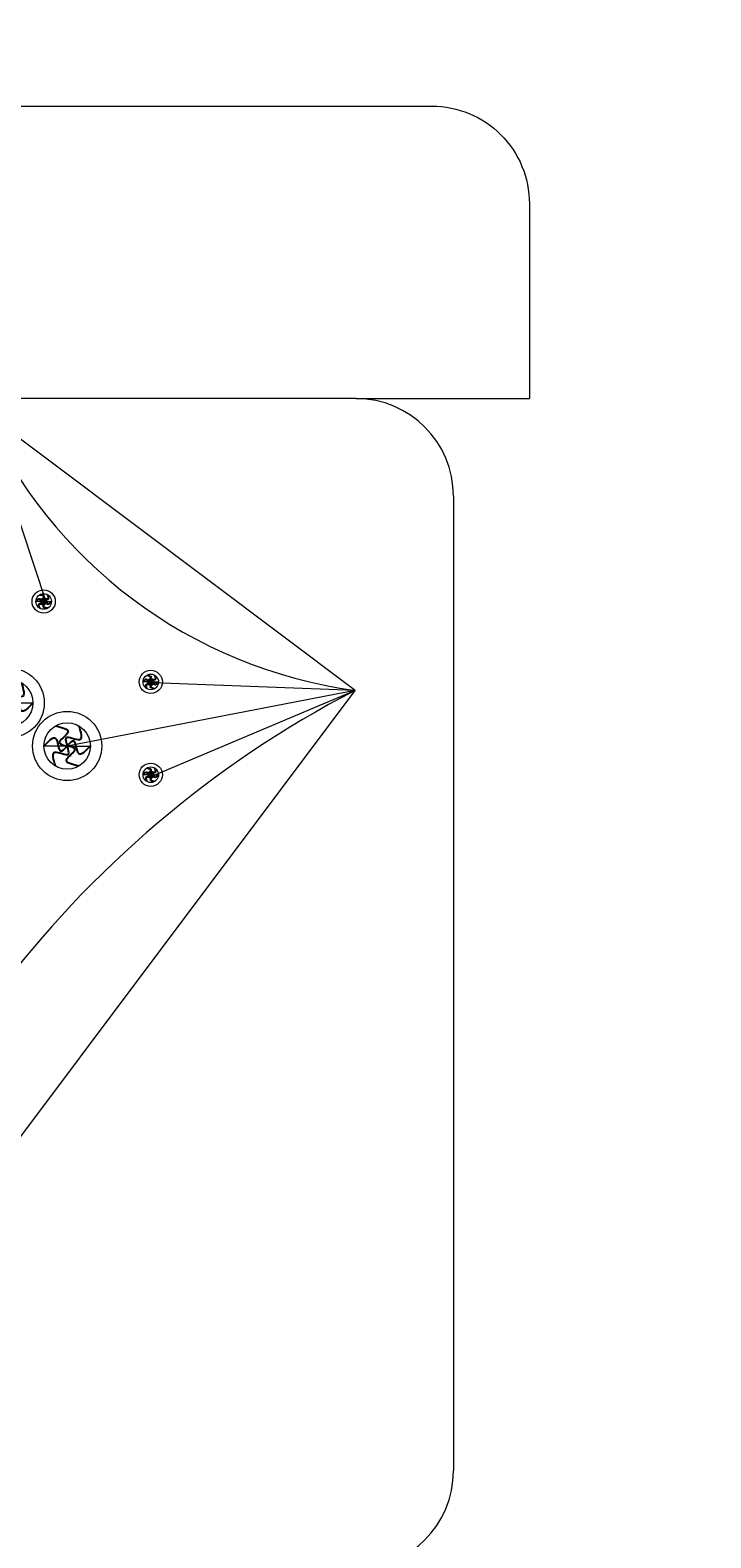
# Model space of a CAD drawing. Units: inches. Extents: x -61 to 1599, y -1316 to 257.
# Tile 105 of 204: x 142 to 156, y -99 to -68. Entities that reach past the tile are written whole.
import ezdxf

# ---------------------------------------------------------------- set-up
doc = ezdxf.new("R2010")
doc.units = ezdxf.units.IN
doc.header["$MEASUREMENT"] = 0
doc.layers.add('A-ANNO-DIMS', color=2, linetype='Continuous', lineweight=18)
doc.layers.add('FURNITURE', color=83, linetype='Continuous', lineweight=18)
doc.layers.add('FUR', color=83, linetype='Continuous')
doc.styles.get("Standard").update_dxf_attribs({"font": 'arial.ttf'})
doc.dimstyles.get("Standard").update_dxf_attribs({"dimtxt": 0.18, "dimasz": 0.18, "dimexe": 0.18, "dimexo": 0.0625, "dimgap": 0.09, "dimtad": 0, "dimtih": 1, "dimtoh": 1, "dimdec": 0, "dimzin": 0, "dimdsep": 46, "dimlunit": 3, "dimtxsty": 'Standard', "dimcen": 0.09, "dimadec": 0, "dimazin": 0, "dimtfac": 1, "dimtdec": 0, "dimtofl": 0, "dimtmove": 0, "dimatfit": 3, "dimfxl": 1, "dimtolj": 1, "dimtzin": 0, "dimarcsym": 0})

# ---------------------------------------------------------------- blocks, each defined once
blk = doc.blocks.new('*U209')
at = {"layer": 'FUR'}
blk.add_open_spline([(0.015, 0.238), (-0.088, 0.143), (-0.292, -0.045), (0.224, -0.053), (0.072, -0.187), (0.015, -0.238)], degree=3, knots=[0, 0, 0, 0, 0.2846533, 0.5662105, 0.736751, 0.736751, 0.736751, 0.736751], dxfattribs=at)
blk = doc.blocks.new('*U188')
at = {"layer": 'FUR', "transparency": 16777216}
blk.add_blockref('*U209', (662.716, -238.357), dxfattribs=at)
for p, rotation in [((662.929, -238.463), 300), ((662.517, -238.489), 60), ((662.531, -238.727), 120), ((662.944, -238.702), 240), ((662.745, -238.833), 180)]:
    blk.add_blockref('*U209', p, dxfattribs=dict(at, rotation=rotation))
blk = doc.blocks.new('*U208')
at = {"layer": 'FUR'}
blk.add_open_spline([(0.005, 0.08), (-0.03, 0.048), (-0.098, -0.015), (0.075, -0.018), (0.024, -0.063), (0.005, -0.08)], degree=3, knots=[0, 0, 0, 0, 0.0954578, 0.1898773, 0.2470677, 0.2470677, 0.2470677, 0.2470677], dxfattribs=at)
blk = doc.blocks.new('*U189')
at = {"layer": 'FUR', "transparency": 16777216}
for p, rotation in [((222.173, -79.977), 60), ((222.178, -80.056), 120), ((222.25, -80.092), 180), ((222.312, -79.968), 300), ((222.317, -80.048), 240)]:
    blk.add_blockref('*U208', p, dxfattribs=dict(at, rotation=rotation))
blk.add_blockref('*U208', (222.24, -79.932), dxfattribs=at)
blk = doc.blocks.new('*U192')
at = {"layer": 'FUR'}
blk.add_open_spline([(0.015, 0.238), (-0.088, 0.143), (-0.292, -0.045), (0.224, -0.053), (0.072, -0.187), (0.015, -0.238)], degree=3, knots=[0, 0, 0, 0, 0.2846533, 0.5662105, 0.736751, 0.736751, 0.736751, 0.736751], dxfattribs=at)
blk = doc.blocks.new('*U193')
at = {"layer": 'FUR', "transparency": 16777216}
blk.add_blockref('*U192', (662.716, -238.357), dxfattribs=at)
for p, rotation in [((662.929, -238.463), 300), ((662.517, -238.489), 60), ((662.531, -238.727), 120), ((662.944, -238.702), 240), ((662.745, -238.833), 180)]:
    blk.add_blockref('*U192', p, dxfattribs=dict(at, rotation=rotation))
blk = doc.blocks.new('*U204')
at = {"layer": 'FUR'}
blk.add_open_spline([(0.005, 0.08), (-0.03, 0.048), (-0.098, -0.015), (0.075, -0.018), (0.024, -0.063), (0.005, -0.08)], degree=3, knots=[0, 0, 0, 0, 0.0954578, 0.1898773, 0.2470677, 0.2470677, 0.2470677, 0.2470677], dxfattribs=at)
blk = doc.blocks.new('*U205')
at = {"layer": 'FUR', "transparency": 16777216}
for p, rotation in [((222.173, -79.977), 60), ((222.178, -80.056), 120), ((222.25, -80.092), 180), ((222.312, -79.968), 300), ((222.317, -80.048), 240)]:
    blk.add_blockref('*U204', p, dxfattribs=dict(at, rotation=rotation))
blk.add_blockref('*U204', (222.24, -79.932), dxfattribs=at)
blk = doc.blocks.new('*U206')
at = {"layer": 'FUR'}
blk.add_open_spline([(0.005, 0.08), (-0.03, 0.048), (-0.098, -0.015), (0.075, -0.018), (0.024, -0.063), (0.005, -0.08)], degree=3, knots=[0, 0, 0, 0, 0.0954578, 0.1898773, 0.2470677, 0.2470677, 0.2470677, 0.2470677], dxfattribs=at)
blk = doc.blocks.new('*U207')
at = {"layer": 'FUR', "transparency": 16777216}
for p, rotation in [((222.173, -79.977), 60), ((222.178, -80.056), 120), ((222.25, -80.092), 180), ((222.312, -79.968), 300), ((222.317, -80.048), 240)]:
    blk.add_blockref('*U206', p, dxfattribs=dict(at, rotation=rotation))
blk.add_blockref('*U206', (222.24, -79.932), dxfattribs=at)
blk = doc.blocks.new('SOFA-LOVESEAT')
for p, q in [((22.442, 54), (5.47, 54)), ((22.442, 54), (26, 54)), ((14.776, 53.751), (16.081, 49.817)), ((24.442, 52), (24.442, 32)), ((16.029, 49.837), (15.869, 49.837)), ((16.029, 49.837), (16.189, 49.837)), ((22.422, 48.013), (16.511, 46.872)), ((18.228, 48.187), (18.068, 48.187)), ((18.228, 48.187), (18.388, 48.187)), ((22.422, 48.013), (18.28, 48.167)), ((22.422, 48.013), (18.28, 46.263)), ((15.332, 47.757), (15.808, 47.757)), ((16.511, 46.872), (16.035, 46.872)), ((16.511, 46.872), (16.988, 46.872)), ((18.228, 46.282), (18.068, 46.282)), ((18.228, 46.282), (18.388, 46.282))]:
    blk.add_line(p, q)
blk.add_lwpolyline([(26, 6), (26, 2, -0.414214), (24, 0), (2, 0, -0.414214), (0, 2), (0, 58, -0.414213), (2, 60), (24, 60, -0.414214), (26, 58), (26, 54)], format="xyb")
blk.add_lwpolyline([(11.116, 32.948), (22.422, 48.013), (14.776, 53.751), (3.47, 38.686)], close=True)
for centre, radius in [((16.029, 49.837), 0.238), ((16.029, 49.837), 0.16), ((15.332, 47.757), 0.71), ((18.228, 48.187), 0.238), ((18.228, 48.187), 0.16), ((15.332, 47.757), 0.476), ((16.511, 46.872), 0.71), ((16.511, 46.872), 0.476), ((18.228, 46.282), 0.238), ((18.228, 46.282), 0.16)]:
    blk.add_circle(centre, radius)
for centre, radius, start, end in [((22.442, 52), 2, 0, 90), ((23.745, 57.74), 9.816, 203.9742, 262.253), ((32.433, 28.726), 21.731, 117.4317, 168.7956), ((22.442, 32), 2, 270, 0)]:
    blk.add_arc(centre, radius, start, end)
at = {"xscale": -1, "rotation": 90.00003000000098}
for name, p in [('*U189', (-63.984, 272.082)), ('*U188', (-223.264, 710.487)), ('*U205', (-61.785, 270.431)), ('*U193', (-222.084, 709.602)), ('*U207', (-61.785, 268.527))]:
    blk.add_blockref(name, p, dxfattribs=at)
blk = doc.blocks.new('*D687')
at = {"layer": 'A-ANNO-DIMS', "color": 0, "lineweight": -2, "transparency": 16777216}
for p, q in [((289.418, 181.677), (-61.077, 181.677)), ((-60.897, 181.497), (-60.897, -528.952)), ((-60.897, -1239.765), (-60.897, -529.316)), ((319.64, -1239.945), (-61.077, -1239.945))]:
    blk.add_line(p, q, dxfattribs=at)
at = {"layer": 'A-ANNO-DIMS', "color": 0, "transparency": 16777216}
for points in [[(-60.927, 181.497), (-60.867, 181.497), (-60.897, 181.677)], [(-60.927, -1239.765), (-60.867, -1239.765), (-60.897, -1239.945)]]:
    blk.add_solid(points, dxfattribs=at)
at = {"layer": 'DEFPOINTS', "color": 0, "transparency": 16777216}
for p in [(289.481, 181.677), (-60.897, -1239.945), (319.703, -1239.945)]:
    blk.add_point(p, dxfattribs=at)
at = {"layer": 'A-ANNO-DIMS', "color": 0, "transparency": 16777216, "insert": (-60.897, -529.134), "char_height": 0.18, "attachment_point": 5}
blk.add_mtext('\\A1;1421.6', dxfattribs=at)
blk = doc.blocks.new('*D700')
at = {"layer": 'A-ANNO-DIMS', "color": 0, "lineweight": -2, "transparency": 16777216}
for p, q in [((14.703, -616.882), (14.703, 257.457)), ((179.752, -616.882), (179.752, 257.457)), ((14.883, 257.277), (96.772, 257.277)), ((179.572, 257.277), (97.683, 257.277))]:
    blk.add_line(p, q, dxfattribs=at)
at = {"layer": 'A-ANNO-DIMS', "color": 0, "transparency": 16777216}
for points in [[(14.883, 257.307), (14.883, 257.247), (14.703, 257.277)], [(179.572, 257.307), (179.572, 257.247), (179.752, 257.277)]]:
    blk.add_solid(points, dxfattribs=at)
at = {"layer": 'DEFPOINTS', "color": 0, "transparency": 16777216}
for p in [(179.752, 257.277), (14.703, -616.945), (179.752, -616.945)]:
    blk.add_point(p, dxfattribs=at)
at = {"layer": 'A-ANNO-DIMS', "color": 0, "transparency": 16777216, "insert": (97.227, 257.277), "char_height": 0.18, "attachment_point": 5}
blk.add_mtext('\\A1;165.05', dxfattribs=at)

msp = doc.modelspace()

# ---------------------------------------------------------------- block references
at = {"layer": 'FURNITURE'}
msp.add_blockref('SOFA-LOVESEAT', (125.901, -129.695), dxfattribs=at)

# ---------------------------------------------------------------- dimensions: what is measured, and where the dimension line sits
at = {"layer": 'A-ANNO-DIMS'}
dim = msp.add_linear_dim(base=(179.7521, 257.2771), p1=(14.7028, -616.9446), p2=(179.7521, -616.9446), dimstyle='Standard', override={"dimdec": 2, "dimlfac": 1, "dimrnd": 0, "dimzin": 0, "dimdsep": 46, "dimlunit": 2}, dxfattribs=at)
dim.commit()
dim.dimension.update_dxf_attribs({"geometry": '*D700', "text_midpoint": (97.2274, 257.2771)})
dim = msp.add_linear_dim(base=(-60.8972, -1239.9446), p1=(289.4807, 181.6771), p2=(319.7028, -1239.9446), angle=90, dimstyle='Standard', override={"dimdec": 1, "dimlfac": 1, "dimrnd": 0, "dimzin": 0, "dimdsep": 46, "dimlunit": 2}, dxfattribs=at)
dim.commit()
dim.dimension.update_dxf_attribs({"geometry": '*D687', "text_midpoint": (-60.8972, -529.1337)})

doc.saveas('drawing.dxf')
